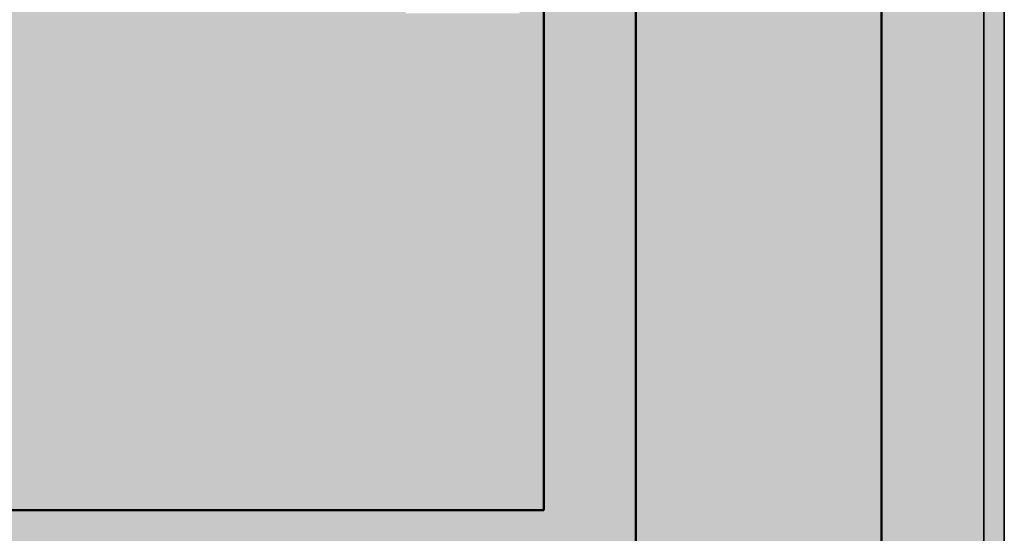
# Model space of a CAD drawing. Units: inches. Extents: x 528 to 2620, y -1066 to 798.
# Tile 13 of 41: x 848 to 944, y 523 to 573. Entities that reach past the tile are written whole.
import ezdxf

# ---------------------------------------------------------------- set-up
doc = ezdxf.new("R2010")
doc.units = ezdxf.units.IN
doc.header["$MEASUREMENT"] = 0
for name, color, linetype, lineweight in [('A-WALL', 7, 'Continuous', 50), ('A-WALL-PATT', 8, 'Continuous', 13), ('C-PROP', 5, 'Continuous', 35)]:
    doc.layers.add(name, color=color, linetype=linetype, lineweight=lineweight)

msp = doc.modelspace()

# ---------------------------------------------------------------- hatches: boundary and pattern name
at = {"layer": 'A-WALL-PATT', "transparency": 33554687}
h = msp.add_hatch(color=256, dxfattribs=at)
h.dxf.hatch_style = 1
h.paths.add_polyline_path([(944.059, 753.922), (584.059, 753.922), (584.059, 208.922), (608.059, 208.922), (608.059, 210.922), (586.059, 210.922), (586.059, 751.922), (942.059, 751.922), (942.059, 210.922), (728.059, 210.922), (728.059, 208.922), (944.059, 208.922)])
h = msp.add_hatch(color=256, dxfattribs=at)
h.dxf.hatch_style = 1
h.paths.add_polyline_path([(942.059, 751.922), (586.059, 751.922), (586.059, 210.922), (608.059, 210.922), (608.059, 220.922), (596.059, 220.922), (596.059, 741.922), (932.059, 741.922), (932.059, 220.922), (770.059, 220.922), (728.059, 220.922), (728.059, 210.922), (942.059, 210.922)])
at = {"layer": 'A-WALL-PATT', "transparency": 33554475}
h = msp.add_hatch(color=256, dxfattribs=at)
h.dxf.hatch_style = 1
h.paths.add_polyline_path([(620.059, 718.922), (908.059, 718.922), (908.059, 268.922), (770.059, 268.922), (770.059, 220.922), (932.059, 220.922), (932.059, 741.922), (596.059, 741.922), (596.059, 391.422), (620.059, 391.422)])
at = {"layer": 'A-WALL-PATT', "transparency": 33554521}
h = msp.add_hatch(color=256, dxfattribs=at)
h.dxf.hatch_style = 1
h.paths.add_polyline_path([(629.059, 709.922), (677.559, 709.922), (677.559, 718.922), (620.059, 718.922), (620.059, 667.922), (629.059, 667.922)])
h.paths.add_polyline_path([(790.559, 718.922), (725.559, 718.922), (725.559, 709.922), (774.059, 709.922), (774.059, 577.922), (768.481, 577.922), (768.559, 573.422), (774.059, 573.422), (774.059, 567.422), (778.559, 567.422), (778.559, 669.422), (831.059, 669.422), (831.059, 675.922), (826.559, 675.922), (826.559, 673.922), (778.559, 673.922), (778.559, 709.922), (790.559, 709.922)])
h.paths.add_polyline_path([(908.059, 718.922), (879.059, 718.922), (879.059, 709.922), (899.059, 709.922), (899.059, 641.672), (908.059, 641.672)])
h.paths.add_polyline_path([(629.059, 619.922), (620.059, 619.922), (620.059, 561.422), (629.059, 561.422), (629.059, 573.422), (724.059, 573.422), (724.059, 569.422), (728.559, 569.422), (728.559, 577.922), (629.059, 577.922)])
h.paths.add_polyline_path([(779.059, 391.422), (779.059, 400.422), (770.059, 400.422), (764.059, 400.422), (764.059, 397.422), (764.059, 391.422), (770.059, 391.422), (770.059, 268.922), (815.059, 268.922), (815.059, 277.922), (779.059, 277.922), (779.059, 359.767)])
h.paths.add_polyline_path([(908.059, 395.922), (899.059, 395.922), (851.059, 395.922), (851.059, 391.422), (899.059, 391.422), (899.059, 277.922), (863.059, 277.922), (863.059, 268.922), (908.059, 268.922)])
h.paths.add_polyline_path([(908.059, 593.672), (899.059, 593.672), (899.059, 525.422), (778.559, 525.422), (778.559, 527.172), (774.059, 527.172), (774.059, 520.922), (899.059, 520.922), (899.059, 443.922), (908.059, 443.922)])
h.paths.add_polyline_path([(629.059, 520.922), (728.559, 520.922), (728.559, 545.422), (724.059, 545.422), (724.059, 525.422), (629.059, 525.422), (629.059, 537.422), (620.059, 537.422), (620.059, 484.672), (629.059, 484.672)])
h.paths.add_polyline_path([(629.059, 436.672), (620.059, 436.672), (620.059, 391.422), (648.559, 391.422), (648.559, 400.422), (629.059, 400.422)])
h.paths.add_polyline_path([(716.059, 397.422), (716.059, 400.422), (696.559, 400.422), (696.559, 391.422), (716.059, 391.422)])
at = {"layer": 'A-WALL-PATT', "transparency": 33554590}
h = msp.add_hatch(color=256, dxfattribs=at)
h.dxf.hatch_style = 1
h.paths.add_polyline_path([(774.059, 709.922), (629.059, 709.922), (629.059, 577.922), (728.559, 577.922), (728.559, 579.422), (728.559, 619.422), (730.309, 619.422), (730.309, 619.384, -0.401453), (768.559, 579.422), (768.559, 577.922), (774.059, 577.922)])
h.paths.add_polyline_path([(723.896, 686.058), (723.968, 686.064), (723.828, 686.128)], flags=0)
h.paths.add_polyline_path([(722.785, 642.699), (722.893, 642.756), (722.893, 684.992), (722.647, 685.244), (722.647, 685.82), (723.079, 686.262), (723.533, 686.262), (723.968, 686.064), (724.739, 686.128), (770.696, 686.128), (770.78, 686.14), (771.126, 686.266), (771.694, 686.094), (771.94, 685.478), (771.67, 684.904), (771.582, 684.871), (771.582, 642.782), (771.878, 642.514), (771.878, 641.921), (771.511, 641.462), (770.855, 641.462), (770.401, 641.833), (770.401, 641.551), (724.739, 641.551), (723.991, 641.705), (723.443, 641.414), (722.879, 641.585), (722.597, 642.142)], flags=16)
h.paths.add_polyline_path([(723.994, 641.704), (723.994, 641.707), (723.991, 641.705)], flags=0)
h.paths.add_polyline_path([(722.893, 642.732), (722.893, 684.992), (722.647, 685.244), (722.647, 685.82), (723.079, 686.262), (723.287, 686.262), (722.991, 686.172), (722.794, 685.971), (722.647, 685.68), (722.647, 685.434), (722.745, 685.143), (722.942, 684.942), (723.238, 684.807), (723.484, 684.807), (723.779, 684.897), (723.976, 685.098), (724.174, 685.488), (724.124, 685.635), (724.124, 685.249), (723.631, 684.746), (723.631, 642.961), (724.124, 642.514), (724.124, 641.887), (723.656, 641.462), (723.079, 641.462), (722.647, 641.904), (722.647, 642.48)], flags=0)
h.paths.add_polyline_path([(722.647, 642.29), (722.647, 642.044), (722.794, 641.753), (723.079, 641.462), (723.287, 641.462), (722.879, 641.585), (722.597, 642.142)], flags=0)
h.paths.add_polyline_path([(770.745, 686.128), (770.58, 686.128), (770.551, 686.057)], flags=0)
h.paths.add_polyline_path([(743.299, 645.288), (753.227, 659.398), (748.69, 663.75), (753.234, 668.538), (743.299, 682.458), (743.791, 682.592), (744.136, 682.681), (744.53, 682.928), (744.628, 683.084), (745.017, 683.327), (744.53, 684.069), (744.776, 684.158), (744.874, 684.315), (745.514, 684.404), (746.081, 684.651), (746.474, 684.651), (746.819, 684.807), (747.459, 685.031), (747.705, 685.143), (748.198, 685.277), (748.394, 685.523), (748.862, 685.523), (749.994, 686.128), (753.488, 676.03), (757.379, 680.153), (757.791, 679.758), (758.044, 680.645), (758.29, 681.227), (758.29, 682.055), (758.019, 682.592), (757.871, 683.174), (757.822, 683.778), (758.388, 684.069), (758.979, 684.203), (759.619, 684.158), (760.21, 683.957), (760.751, 683.666), (761.859, 683.666), (762.401, 683.957), (762.991, 684.114), (763.631, 684.114), (764.198, 683.957), (764.739, 683.666), (766.118, 683.666), (766.659, 683.957), (767.25, 684.158), (767.865, 684.203), (768.456, 684.069), (769.047, 683.778), (768.998, 683.174), (768.85, 682.592), (768.554, 682.055), (768.554, 681.227), (768.801, 680.645), (769.092, 679.75), (768.948, 678.832), (768.801, 678.228), (768.554, 677.646), (768.554, 676.818), (768.801, 676.237), (769.092, 675.341), (768.948, 674.424), (768.801, 673.82), (768.554, 673.283), (768.554, 672.41), (768.801, 671.873), (768.998, 671.291), (769.047, 670.642), (768.948, 670.016), (768.801, 669.411), (768.554, 668.874), (768.554, 668.002), (768.974, 667.239), (769.047, 666.279), (769.047, 665.563), (768.456, 665.316), (767.865, 665.16), (767.25, 665.16), (766.659, 665.361), (766.118, 665.697), (764.739, 665.697), (763.945, 665.204), (762.991, 665.204), (762.401, 665.361), (761.859, 665.697), (761.005, 665.697), (762.696, 664.086), (760.741, 662.027), (761.859, 662.027), (762.401, 662.318), (763.342, 662.548), (764.247, 662.318), (764.788, 662.027), (766.118, 662.027), (766.659, 662.318), (767.25, 662.519), (767.865, 662.564), (768.505, 662.43), (769.047, 662.116), (769.047, 661.4), (769.047, 660.796), (768.85, 660.214), (768.554, 659.677), (768.554, 658.849), (768.85, 658.267), (768.998, 657.663), (769.069, 656.749), (768.85, 655.851), (768.554, 655.269), (768.554, 654.441), (768.85, 653.859), (769.069, 652.961), (768.998, 652.046), (768.85, 651.442), (768.554, 650.905), (768.554, 650.032), (768.85, 649.495), (768.998, 648.914), (769.047, 648.265), (768.998, 647.638), (768.85, 647.034), (768.554, 646.497), (768.554, 645.624), (768.85, 645.087), (769.047, 644.55), (769.047, 643.901), (768.505, 643.655), (767.865, 643.521), (767.25, 643.521), (766.659, 643.722), (766.118, 644.058), (764.788, 644.058), (764.247, 643.722), (763.342, 643.492), (762.401, 643.722), (761.859, 644.058), (760.801, 644.058), (760.259, 643.722), (759.668, 643.521), (759.028, 643.521), (758.388, 643.655), (757.871, 643.901), (757.871, 644.55), (758.044, 645.087), (758.339, 645.624), (758.339, 646.497), (758.044, 647.034), (757.921, 647.638), (757.866, 648.059), (757.379, 647.593), (753.422, 651.773), (749.994, 641.618), (749.502, 641.708), (749.354, 641.954), (748.542, 642.446), (747.311, 642.939), (746.652, 642.939), (746.327, 643.185), (745.514, 643.565), (744.53, 643.655), (745.011, 644.4), (744.628, 644.639), (744.136, 644.886), (743.791, 645.132)], flags=0)
h.paths.add_polyline_path([(755.656, 654.933), (756.542, 654.687), (757.527, 654.329), (756.641, 654.575)], flags=0)
h.paths.add_polyline_path([(758.339, 649.204), (758.339, 648.712), (758.585, 644.304), (758.585, 648.802)], flags=0)
h.paths.add_polyline_path([(758.339, 649.294), (758.093, 649.697), (758.359, 649.165)], flags=0)
h.paths.add_polyline_path([(755.656, 672.79), (756.493, 673.037), (757.358, 673.351), (757.353, 673.358), (756.641, 673.149)], flags=0)
h.paths.add_polyline_path([(760.264, 639.641), (771.408, 639.641), (771.408, 624.039), (760.264, 624.039)], flags=16)
h.paths.add_polyline_path([(761.378, 638.526), (770.294, 638.526), (770.294, 625.153), (761.378, 625.153)], flags=0)
edge = h.paths.add_edge_path(flags=0)
edge.add_ellipse((765.836, 631.84), major_axis=(-2.245, 2.245), ratio=1, start_angle=-45, end_angle=45, ccw=False)
edge.add_ellipse((765.836, 631.84), major_axis=(-2.245, 2.245), ratio=1, start_angle=-135, end_angle=-45, ccw=False)
edge.add_ellipse((765.836, 631.84), major_axis=(-2.245, 2.245), ratio=1, start_angle=135, end_angle=-135, ccw=False)
edge.add_ellipse((765.836, 631.84), major_axis=(-2.245, 2.245), ratio=1, start_angle=45, end_angle=135, ccw=False)
h.paths.add_polyline_path([(758.585, 683.42), (758.585, 678.922), (758.373, 678.575), (758.339, 678.43), (758.093, 678.049), (758.339, 678.519), (758.339, 679.011)], flags=0)
h.paths.add_polyline_path([(760.264, 688.038), (760.264, 703.64), (771.408, 703.64), (771.408, 688.038)], flags=16)
h.paths.add_polyline_path([(770.401, 685.389), (770.401, 685.846), (770.855, 686.217), (771.511, 686.217), (771.878, 685.758), (771.878, 685.165), (771.582, 684.897), (771.582, 642.782), (771.878, 642.514), (771.878, 641.921), (771.511, 641.462), (770.855, 641.462), (770.401, 641.833), (770.401, 642.29)], flags=0)
h.paths.add_polyline_path([(770.532, 642.678), (771.052, 643.009), (771.67, 642.775), (771.94, 642.201), (771.694, 641.585), (771.126, 641.413), (770.551, 641.622), (770.347, 642.132)], flags=16)
h.paths.add_polyline_path([(761.378, 689.152), (761.378, 702.526), (770.294, 702.526), (770.294, 689.152)], flags=0)
edge = h.paths.add_edge_path(flags=0)
edge.add_ellipse((765.836, 695.839), major_axis=(2.245, 2.245), ratio=1, start_angle=405, end_angle=495, ccw=False)
edge.add_ellipse((765.836, 695.839), major_axis=(2.245, 2.245), ratio=1, start_angle=675, end_angle=765, ccw=False)
edge.add_ellipse((765.836, 695.839), major_axis=(2.245, 2.245), ratio=1, start_angle=585, end_angle=675, ccw=False)
edge.add_ellipse((765.836, 695.839), major_axis=(2.245, 2.245), ratio=1, start_angle=495, end_angle=585, ccw=False)
h.paths.add_polyline_path([(770.696, 684.897), (770.942, 684.74), (771.41, 684.74), (771.73, 685.031), (771.878, 685.344), (771.878, 685.635), (771.694, 686.094), (771.582, 686.128), (771.878, 685.758), (771.878, 685.165), (771.41, 684.74), (770.849, 684.74)], flags=0)
h.paths.add_polyline_path([(899.059, 709.922), (831.059, 709.922), (831.059, 699.922), (829.809, 699.922), (829.809, 675.922), (831.059, 675.922), (831.059, 669.422), (778.559, 669.422), (778.559, 567.172), (780.059, 567.172), (820.059, 567.172), (820.059, 565.422), (820.021, 565.422, -0.401453), (780.059, 527.172), (778.559, 527.172), (778.559, 525.422), (899.059, 525.422)])
h.paths.add_polyline_path([(849.197, 636.014), (849.269, 636.02), (849.129, 636.084)], flags=0)
h.paths.add_polyline_path([(848.193, 634.948), (847.947, 635.2), (847.947, 635.776), (848.379, 636.218), (848.833, 636.218), (849.269, 636.02), (850.039, 636.084), (895.996, 636.084), (896.081, 636.096), (896.426, 636.222), (896.995, 636.05), (897.241, 635.434), (896.97, 634.86), (896.883, 634.827), (896.883, 592.738), (897.178, 592.47), (897.178, 591.877), (896.811, 591.418), (896.155, 591.418), (895.701, 591.789), (895.701, 591.507), (850.039, 591.507), (849.292, 591.661), (848.744, 591.37), (848.18, 591.541), (847.897, 592.098), (848.086, 592.655), (848.193, 592.712)], flags=16)
h.paths.add_polyline_path([(849.294, 591.66), (849.295, 591.663), (849.292, 591.661)], flags=16)
h.paths.add_polyline_path([(848.193, 634.948), (847.947, 635.2), (847.947, 635.776), (848.379, 636.218), (848.587, 636.218), (848.292, 636.128), (848.095, 635.927), (847.947, 635.636), (847.947, 635.39), (848.046, 635.099), (848.243, 634.897), (848.538, 634.763), (848.784, 634.763), (849.079, 634.853), (849.276, 635.054), (849.474, 635.444), (849.424, 635.591), (849.424, 635.205), (848.932, 634.702), (848.932, 592.917), (849.424, 592.47), (849.424, 591.843), (848.956, 591.418), (848.379, 591.418), (847.947, 591.86), (847.947, 592.436), (848.193, 592.688)], flags=0)
h.paths.add_polyline_path([(847.947, 592.246), (847.947, 592), (848.095, 591.709), (848.379, 591.418), (848.587, 591.418), (848.18, 591.541), (847.897, 592.098)], flags=16)
h.paths.add_polyline_path([(896.046, 636.084), (895.88, 636.084), (895.852, 636.013)], flags=0)
h.paths.add_polyline_path([(868.599, 632.414), (869.092, 632.548), (869.436, 632.637), (869.83, 632.884), (869.929, 633.04), (870.318, 633.283), (869.83, 634.025), (870.076, 634.114), (870.175, 634.271), (870.815, 634.36), (871.381, 634.607), (871.775, 634.607), (872.119, 634.763), (872.759, 634.987), (873.006, 635.099), (873.498, 635.233), (873.695, 635.479), (874.163, 635.479), (875.295, 636.084), (878.788, 625.986), (882.679, 630.109), (883.091, 629.714), (883.344, 630.601), (883.59, 631.183), (883.59, 632.011), (883.319, 632.548), (883.172, 633.13), (883.123, 633.734), (883.689, 634.025), (884.279, 634.159), (884.919, 634.114), (885.51, 633.913), (886.052, 633.622), (887.159, 633.622), (887.701, 633.913), (888.292, 634.07), (888.932, 634.07), (889.498, 633.913), (890.039, 633.622), (891.418, 633.622), (891.959, 633.913), (892.55, 634.114), (893.166, 634.159), (893.756, 634.025), (894.347, 633.734), (894.298, 633.13), (894.15, 632.548), (893.855, 632.011), (893.855, 631.183), (894.101, 630.601), (894.393, 629.706), (894.249, 628.788), (894.101, 628.184), (893.855, 627.602), (893.855, 626.774), (894.101, 626.193), (894.393, 625.297), (894.249, 624.38), (894.101, 623.776), (893.855, 623.239), (893.855, 622.366), (894.101, 621.829), (894.298, 621.247), (894.347, 620.598), (894.249, 619.972), (894.101, 619.367), (893.855, 618.83), (893.855, 617.958), (894.274, 617.195), (894.347, 616.235), (894.347, 615.518), (893.756, 615.272), (893.166, 615.116), (892.55, 615.116), (891.959, 615.317), (891.418, 615.653), (890.039, 615.653), (889.245, 615.16), (888.292, 615.16), (887.701, 615.317), (887.159, 615.653), (886.305, 615.653), (887.996, 614.042), (886.041, 611.983), (887.159, 611.983), (887.701, 612.274), (888.642, 612.504), (889.547, 612.274), (890.089, 611.983), (891.418, 611.983), (891.959, 612.274), (892.55, 612.475), (893.166, 612.52), (893.806, 612.386), (894.347, 612.072), (894.347, 611.356), (894.347, 610.752), (894.15, 610.17), (893.855, 609.633), (893.855, 608.805), (894.15, 608.223), (894.298, 607.619), (894.37, 606.705), (894.15, 605.807), (893.855, 605.225), (893.855, 604.397), (894.15, 603.815), (894.37, 602.917), (894.298, 602.002), (894.15, 601.398), (893.855, 600.861), (893.855, 599.988), (894.15, 599.451), (894.298, 598.87), (894.347, 598.221), (894.298, 597.594), (894.15, 596.99), (893.855, 596.453), (893.855, 595.58), (894.15, 595.043), (894.347, 594.506), (894.347, 593.857), (893.806, 593.611), (893.166, 593.477), (892.55, 593.477), (891.959, 593.678), (891.418, 594.014), (890.089, 594.014), (889.547, 593.678), (888.642, 593.448), (887.701, 593.678), (887.159, 594.014), (886.101, 594.014), (885.559, 593.678), (884.969, 593.477), (884.329, 593.477), (883.689, 593.611), (883.172, 593.857), (883.172, 594.506), (883.344, 595.043), (883.639, 595.58), (883.639, 596.453), (883.344, 596.99), (883.221, 597.594), (883.167, 598.015), (882.679, 597.549), (878.722, 601.729), (875.295, 591.574), (874.803, 591.664), (874.655, 591.91), (873.843, 592.402), (872.612, 592.895), (871.952, 592.895), (871.627, 593.141), (870.815, 593.521), (869.83, 593.611), (870.311, 594.356), (869.929, 594.595), (869.436, 594.842), (869.092, 595.088), (868.599, 595.244), (878.528, 609.354), (873.99, 613.706), (878.535, 618.494)], flags=0)
h.paths.add_polyline_path([(880.956, 622.746), (881.793, 622.993), (882.659, 623.307), (882.654, 623.314), (881.941, 623.104)], flags=0)
h.paths.add_polyline_path([(880.956, 604.889), (881.843, 604.643), (882.827, 604.285), (881.941, 604.531)], flags=16)
h.paths.add_polyline_path([(883.393, 628.005), (883.639, 628.475), (883.639, 628.967), (883.886, 633.376), (883.886, 628.878), (883.674, 628.531), (883.639, 628.386)], flags=0)
h.paths.add_polyline_path([(883.639, 599.16), (883.639, 598.668), (883.886, 594.26), (883.886, 598.758)], flags=16)
h.paths.add_polyline_path([(883.639, 599.25), (883.393, 599.653), (883.659, 599.121)], flags=16)
h.paths.add_polyline_path([(885.564, 637.994), (885.564, 653.596), (896.709, 653.596), (896.709, 637.994)], flags=16)
h.paths.add_polyline_path([(885.564, 589.597), (896.709, 589.597), (896.709, 573.995), (885.564, 573.995)], flags=16)
h.paths.add_polyline_path([(886.679, 639.108), (886.679, 652.482), (895.594, 652.482), (895.594, 639.108)], flags=0)
h.paths.add_polyline_path([(886.679, 588.482), (895.594, 588.482), (895.594, 575.109), (886.679, 575.109)], flags=0)
edge = h.paths.add_edge_path(flags=0)
edge.add_ellipse((891.136, 645.795), major_axis=(2.245, 2.245), ratio=1, start_angle=405, end_angle=495, ccw=False)
edge.add_ellipse((891.136, 645.795), major_axis=(2.245, 2.245), ratio=1, start_angle=675, end_angle=765, ccw=False)
edge.add_ellipse((891.136, 645.795), major_axis=(2.245, 2.245), ratio=1, start_angle=585, end_angle=675, ccw=False)
edge.add_ellipse((891.136, 645.795), major_axis=(2.245, 2.245), ratio=1, start_angle=495, end_angle=585, ccw=False)
edge = h.paths.add_edge_path(flags=0)
edge.add_ellipse((891.136, 581.796), major_axis=(-2.245, 2.245), ratio=1, start_angle=-45, end_angle=45, ccw=False)
edge.add_ellipse((891.136, 581.796), major_axis=(-2.245, 2.245), ratio=1, start_angle=-135, end_angle=-45, ccw=False)
edge.add_ellipse((891.136, 581.796), major_axis=(-2.245, 2.245), ratio=1, start_angle=135, end_angle=-135, ccw=False)
edge.add_ellipse((891.136, 581.796), major_axis=(-2.245, 2.245), ratio=1, start_angle=45, end_angle=135, ccw=False)
h.paths.add_polyline_path([(895.701, 635.345), (895.701, 635.802), (896.155, 636.173), (896.811, 636.173), (897.178, 635.714), (897.178, 635.121), (896.883, 634.853), (896.883, 592.738), (897.178, 592.47), (897.178, 591.877), (896.811, 591.418), (896.155, 591.418), (895.701, 591.789), (895.701, 592.246)], flags=0)
h.paths.add_polyline_path([(895.996, 634.853), (896.243, 634.696), (896.71, 634.696), (897.03, 634.987), (897.178, 635.3), (897.178, 635.591), (896.995, 636.05), (896.883, 636.084), (897.178, 635.714), (897.178, 635.121), (896.71, 634.696), (896.15, 634.696)], flags=0)
h.paths.add_polyline_path([(895.832, 592.634), (896.353, 592.965), (896.97, 592.731), (897.241, 592.157), (896.995, 591.541), (896.426, 591.369), (895.852, 591.578), (895.648, 592.088)], flags=16)
h.paths.add_polyline_path([(725.255, 569.422), (724.059, 569.422), (724.059, 573.422), (629.059, 573.422), (629.059, 525.422), (724.059, 525.422), (724.059, 545.422), (725.255, 545.422)])
h.paths.add_polyline_path([(820.021, 565.422), (780.059, 565.422), (780.059, 567.172), (774.059, 567.172), (774.059, 567.422), (774.059, 573.422), (768.559, 573.422), (768.481, 577.922), (768.559, 577.922), (768.559, 579.422, 0.401453), (730.309, 619.384), (730.309, 579.422), (728.559, 579.422), (728.559, 573.422), (728.559, 569.422), (727.255, 569.422), (727.255, 545.422), (728.559, 545.422), (728.559, 520.922), (665.059, 520.922), (665.059, 436.422), (716.059, 436.422), (716.059, 421.422), (717.809, 421.422), (717.809, 421.358, -0.392996), (740.059, 397.422, -0.392996), (762.309, 421.358), (762.309, 421.422), (764.059, 421.422), (764.059, 400.422), (770.059, 400.422), (779.059, 400.422), (779.059, 391.422), (779.059, 359.767), (795.432, 359.767), (795.432, 294.295), (893.669, 294.295), (893.669, 277.922), (899.059, 277.922), (899.059, 391.422), (851.059, 391.422), (851.059, 395.922), (899.059, 395.922), (899.059, 443.922), (899.059, 520.922), (774.059, 520.922), (774.059, 527.172), (778.559, 527.172), (780.059, 527.172, 0.401453)])
h.paths.add_polyline_path([(774.059, 519.657), (842.122, 519.657), (842.122, 505.072), (788.644, 505.072), (788.644, 474.079), (788.644, 470.433, -0.883215), (779.529, 456.663), (774.971, 456.663, -0.414214), (774.059, 457.575)], flags=16)
h.paths.add_polyline_path([(775.883, 517.834), (840.299, 517.834), (840.299, 514.188), (788.644, 514.188), (788.644, 484.41), (779.529, 484.41), (779.529, 474.079), (775.883, 474.079)], flags=0)
h.paths.add_polyline_path([(706.7, 501.564, -0.254069), (706.7, 493.021), (698.31, 492.555), (698.31, 502.031)], flags=16)
h.paths.add_polyline_path([(691.334, 515.692), (691.8, 507.301), (682.325, 507.301), (682.791, 515.692, -0.254069)], flags=16)
h.paths.add_polyline_path([(695.485, 504.685), (695.485, 479.416), (678.64, 479.416), (678.64, 504.685)], flags=16)
h.paths.add_polyline_path([(706.7, 489.602, -0.254069), (706.7, 481.058), (698.31, 480.592), (698.31, 490.068)], flags=16)
h.paths.add_polyline_path([(675.815, 502.031), (675.815, 492.555), (667.425, 493.021, -0.254069), (667.425, 501.564)], flags=16)
h.paths.add_polyline_path([(691.8, 476.8), (691.334, 468.409, -0.254069), (682.791, 468.409), (682.325, 476.8)], flags=16)
h.paths.add_polyline_path([(675.815, 490.068), (675.815, 480.592), (667.425, 481.058, -0.254069), (667.425, 489.602)], flags=16)
h.paths.add_polyline_path([(764.059, 397.422), (762.309, 397.422), (762.309, 421.358, 0.392996), (740.059, 397.422, 0.392996), (717.809, 421.358), (717.809, 397.422), (716.059, 397.422), (716.059, 391.422), (716.059, 385.422), (764.059, 385.422), (764.059, 391.422)], flags=17)
h.paths.add_polyline_path([(716.059, 436.422), (705.859, 436.422), (705.859, 418.422), (716.059, 418.422), (716.059, 421.422)], flags=17)
h.paths.add_polyline_path([(716.059, 418.422), (705.859, 418.422), (705.859, 400.422), (716.059, 400.422)], flags=17)
h.paths.add_polyline_path([(705.859, 418.422), (695.659, 418.422), (695.659, 400.422), (696.559, 400.422), (705.859, 400.422)], flags=17)
h.paths.add_polyline_path([(705.859, 436.422), (695.659, 436.422), (695.659, 418.422), (705.859, 418.422)], flags=17)
h.paths.add_polyline_path([(695.659, 418.422), (685.459, 418.422), (685.459, 400.422), (695.659, 400.422)], flags=17)
h.paths.add_polyline_path([(695.659, 436.422), (685.459, 436.422), (685.459, 418.422), (695.659, 418.422)], flags=17)
h.paths.add_polyline_path([(685.459, 418.422), (675.259, 418.422), (675.259, 400.422), (685.459, 400.422)], flags=17)
h.paths.add_polyline_path([(685.459, 436.422), (675.259, 436.422), (675.259, 418.422), (685.459, 418.422)], flags=17)
h.paths.add_polyline_path([(675.259, 436.422), (665.059, 436.422), (665.059, 418.422), (675.259, 418.422)])
h.paths.add_polyline_path([(675.259, 418.422), (665.059, 418.422), (665.059, 400.422), (675.259, 400.422)])
h.paths.add_polyline_path([(665.059, 418.422), (646.967, 418.422), (646.991, 436.422), (629.059, 436.422), (629.059, 400.422), (665.059, 400.422)])
h.paths.add_polyline_path([(665.059, 436.422), (646.991, 436.422), (646.967, 418.422), (665.059, 418.422)], flags=17)
h.paths.add_polyline_path([(647.005, 446.622), (629.059, 446.622), (629.059, 436.672), (629.059, 436.422), (646.991, 436.422)])
h.paths.add_polyline_path([(665.059, 446.622), (647.005, 446.622), (646.991, 436.422), (665.059, 436.422)])
h.paths.add_polyline_path([(647.019, 456.822), (629.059, 456.822), (629.059, 446.622), (647.005, 446.622)])
h.paths.add_polyline_path([(665.059, 456.822), (647.019, 456.822), (647.005, 446.622), (665.059, 446.622)])
h.paths.add_polyline_path([(647.032, 467.022), (629.059, 467.022), (629.059, 456.822), (647.019, 456.822)])
h.paths.add_polyline_path([(665.059, 467.022), (647.032, 467.022), (647.019, 456.822), (665.059, 456.822)])
h.paths.add_polyline_path([(665.059, 477.222), (647.046, 477.222), (647.032, 467.022), (665.059, 467.022)])
h.paths.add_polyline_path([(647.046, 477.222), (629.059, 477.222), (629.059, 467.022), (647.032, 467.022)])
h.paths.add_polyline_path([(647.059, 487.222), (629.059, 487.222), (629.059, 477.222), (647.046, 477.222), (647.048, 479.019), (645.53, 483.246), (640.877, 480.371)])
h.paths.add_polyline_path([(665.059, 520.922), (629.059, 520.922), (629.059, 487.222), (647.059, 487.222), (665.059, 487.222)])
h.paths.add_polyline_path([(665.059, 487.222), (647.059, 487.222), (653.224, 480.355), (648.578, 483.242), (647.048, 479.019), (647.046, 477.222), (665.059, 477.222)])

# ---------------------------------------------------------------- linework, layer by layer
at = {"layer": 'A-WALL'}
for p, q in [((932.059, 220.922), (932.059, 741.922)), ((908.059, 268.922), (908.059, 718.922)), ((899.059, 525.422), (899.059, 709.922)), ((899.059, 525.422), (778.559, 525.422))]:
    msp.add_line(p, q, dxfattribs=at)
at = {"layer": 'C-PROP'}
for points in [[(728.059, 208.922), (944.059, 208.922), (944.059, 753.922), (584.059, 753.922), (584.059, 208.922), (608.059, 208.922)], [(728.059, 210.922), (942.059, 210.922), (942.059, 751.922), (586.059, 751.922), (586.059, 210.922), (608.059, 210.922)]]:
    msp.add_lwpolyline(points, dxfattribs=at)
msp.add_lwpolyline([(596.059, 741.922), (596.059, 220.922), (932.059, 220.922), (932.059, 741.922)], close=True, dxfattribs=at)

doc.saveas('drawing.dxf')
